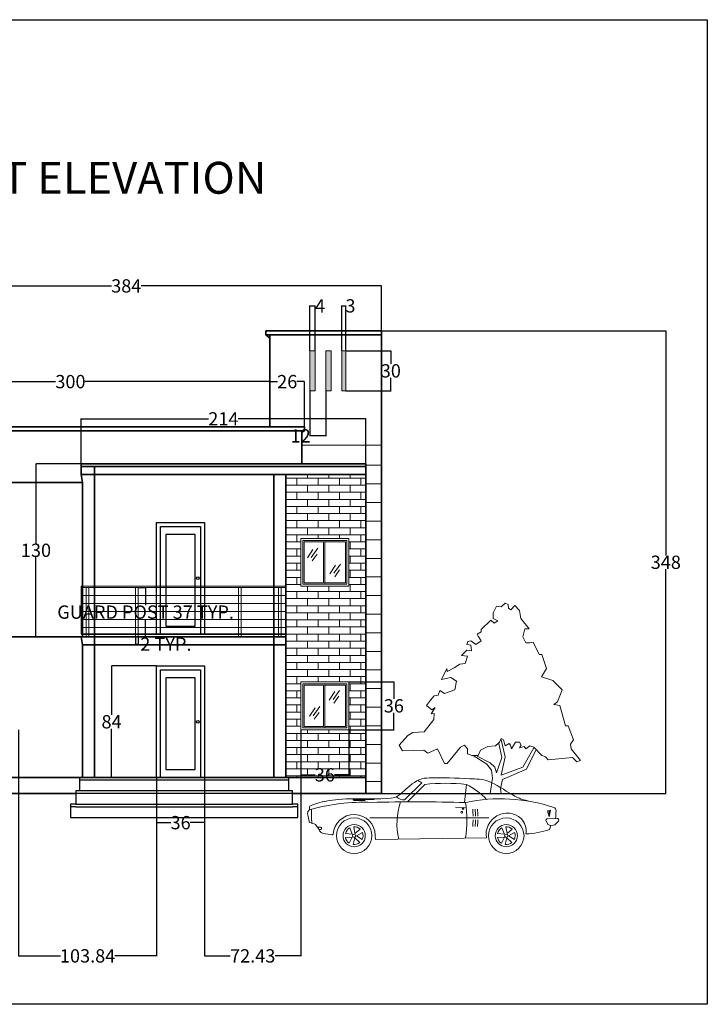
# Model space of a CAD drawing. Units: inches. Extents: x -16 to 1298, y 3 to 744.
# Tile 5 of 5: x 781 to 1298, y 3 to 744. Entities that reach past the tile are written whole.
import ezdxf

# ---------------------------------------------------------------- set-up
doc = ezdxf.new("R2010")
doc.units = ezdxf.units.IN
doc.header["$MEASUREMENT"] = 0
for name, color, linetype, lineweight in [('A-ANNO-DIMS', 2, 'Continuous', 18), ('A-ANNO-TITL', 7, 'Continuous', 35), ('A-DOOR', 3, 'Continuous', 25), ('A-ELEV', 7, 'Continuous', 35), ('A-ELEV-JNTS', 8, 'Continuous', 13), ('A-ELEV-VENT', 7, 'Continuous', 18), ('A-FLOR-HRAL', 4, 'Continuous', 18), ('A-FLOR-STRS', 7, 'Continuous', 25), ('A-GLAZ', 4, 'Continuous', 18), ('A-ROOF', 7, 'Continuous', 35), ('A-SITE-ENTG', 8, 'Continuous', 13), ('C-TOPO', 7, 'Continuous', 30), ('PLANT', 3, 'Continuous', 13)]:
    doc.layers.add(name, color=color, linetype=linetype, lineweight=lineweight)
doc.layers.add('A-ELEV-VENT-PATT', color=18, linetype='Continuous', lineweight=13, true_color=0x000000)
doc.layers.add('A-WALL-PATT', color=251, linetype='Continuous', lineweight=13, true_color=0x636466)
doc.styles.get("Standard").update_dxf_attribs({"font": 'arial.ttf'})
doc.dimstyles.get("Standard").update_dxf_attribs({"dimtxt": 10, "dimasz": 0.18, "dimexe": 0.18, "dimexo": 0.0625, "dimgap": 0.09, "dimtad": 0, "dimtih": 1, "dimtoh": 1, "dimdec": 0, "dimzin": 0, "dimdsep": 46, "dimlunit": 3, "dimtxsty": 'Standard', "dimcen": 0.09, "dimadec": 0, "dimazin": 0, "dimtfac": 1, "dimtdec": 0, "dimtofl": 0, "dimtmove": 0, "dimatfit": 3, "dimfxl": 1, "dimtolj": 1, "dimtzin": 0, "dimarcsym": 0})
pattern_1 = [(0, (565.852, -507.463), (0, 5.334), []), (90, (565.852, -507.463), (-8, 5.334), [5.334, -5.334])]

# ---------------------------------------------------------------- blocks, each defined once
blk = doc.blocks.new('*U12')
for p, q in [((1.5, 1.5), (1.5, 34.5)), ((1.5, 34.5), (18, 34.5)), ((18, 1.5), (18, 34.5)), ((18, 34.5), (34.5, 34.5)), ((34.5, 34.5), (34.5, 1.5)), ((18, 1.5), (1.5, 1.5)), ((34.5, 1.5), (18, 1.5))]:
    blk.add_line(p, q)
blk.add_lwpolyline([(0, 0), (0, 36), (36, 36), (36, 0)], close=True)
for points in [[(17, 33.5), (17, 2.5), (2.5, 2.5), (2.5, 33.5), (17, 33.5)], [(18, 33.5), (33.5, 33.5), (33.5, 2.5), (18, 2.5)]]:
    blk.add_lwpolyline(points)
blk = doc.blocks.new('*U16')
blk.add_lwpolyline([(3.12, 0.01), (0.12, 0.01), (0.12, 84.01), (36.12, 84.01), (36.12, 0.01), (33.12, 0.01)])
for points in [[(33.12, 80.99), (33.12, 0.01), (3.12, 0.01), (3.12, 80.99)], [(29.12, 6.01), (29.12, 74.99), (7.12, 74.99), (7.12, 6.01)]]:
    blk.add_lwpolyline(points, close=True)
blk.add_circle((31.12, 42.01), 1)
blk = doc.blocks.new('*U15')
blk.add_lwpolyline([(3.12, 0.01), (0.12, 0.01), (0.12, 84.01), (36.12, 84.01), (36.12, 0.01), (33.12, 0.01)])
for points in [[(33.12, 80.99), (33.12, 0.01), (3.12, 0.01), (3.12, 80.99)], [(29.12, 6.01), (29.12, 74.99), (7.12, 74.99), (7.12, 6.01)]]:
    blk.add_lwpolyline(points, close=True)
blk.add_circle((31.12, 42.01), 1)
blk = doc.blocks.new('Tree - type 3 evergreen elevation')
for points in [[(22.0124, 137.721), (18.5475, 141.5624), (15.5282, 138.2446), (13.8028, 139.3505), (13.3714, 142.1153), (11.2148, 143.2214), (8.1954, 140.4564), (4.7447, 141.0094), (2.1567, 136.0326), (2.1567, 131.6088), (5.6074, 129.9499), (3.0193, 128.2909), (0.4313, 130.5029), (-6.9015, 123.3141), (-6.9015, 121.6552), (-9.9208, 119.9963), (-9.0581, 118.3373), (-6.9015, 115.0195), (-10.7835, 112.2546), (-14.6656, 115.0195), (-16.8222, 114.4665), (-17.6849, 112.2546), (-14.6656, 111.7016), (-14.2342, 107.2778), (-17.6065, 107.8307), (-21.5669, 103.9599), (-17.2536, 103.4069), (-18.9789, 97.8771), (-22.8609, 97.3241), (-27.1743, 94.5593), (-32.3504, 91.7944), (-32.7817, 94.0063), (-36.6638, 85.7116), (-29.7624, 87.3705), (-25.449, 84.6056), (-26.743, 77.9699), (-34.507, 75.205), (-37.9578, 77.4169), (-39.2518, 74.099), (-42.2711, 73.5461), (-44.8592, 70.2282), (-47.8786, 66.3574), (-43.9965, 63.0395), (-41.4085, 64.6985), (-44.3346, 59.8898), (-42.2089, 60.1377), (-42.5159, 55.7849), (-49.6039, 46.4502), (-58.2307, 45.8972), (-62.1127, 43.6853), (-68.5828, 36.4966), (-65.9947, 32.0727), (-50.0352, 32.6257), (-47.0159, 30.4138), (-39.6831, 33.7317), (-34.507, 22.6721), (-32.3504, 22.6721), (-22.4296, 34.8376), (-19.4102, 36.4966), (-17.2536, 33.7317), (-17.2536, 29.8608), (-13.8028, 28.7549), (-9.0581, 28.7549), (-7.3328, 32.6257), (-1.7254, 35.3906), (3.8821, 35.9436), (6.4701, 38.1555), (6.9014, 38.7085), (8.1954, 41.4734), (9.9208, 40.3674), (11.2148, 35.9436), (14.2341, 37.6025), (15.0968, 36.4966), (15.9595, 33.7317), (18.9789, 38.7085), (21.9982, 38.7085), (23.2922, 36.4966), (21.9982, 34.2847), (25.4489, 35.3906), (26.743, 33.7317), (29.7623, 35.9436), (32.7817, 34.8376), (38.8204, 28.7549), (41.4084, 27.6489), (43.5651, 25.437), (61.6813, 27.0959), (65.132, 23.7781), (67.7201, 24.884), (60.8186, 33.7317), (60.3873, 37.0495), (62.544, 40.3674), (58.662, 50.874), (56.5053, 50.874), (52.1919, 66.3574), (47.8785, 66.9103), (50.4665, 69.1222), (53.9172, 77.9699), (47.0158, 85.1586), (38.3891, 87.9235), (42.2711, 94.0063)], [(42.2711, 94.0063), (38.8204, 104.5129), (36.6637, 104.5129), (32.3503, 113.9135), (29.7623, 113.3605), (26.743, 113.3605), (24.5862, 117.7844), (25.8802, 123.8671), (29.331, 123.8671), (22.8609, 131.6088), (21.9982, 137.6916)], [(-9.9208, 28.2019), (0, 23.2251), (3.4507, 19.9072), (4.7447, 15.4834), (8.6267, 27.0959), (6.4701, 37.6025)], [(8.1954, 40.3674), (11.2148, 27.6489), (8.1954, 13.8245), (24.5862, 19.9072), (32.7817, 34.2847)], [(34.5071, 33.1787), (27.1743, 18.2483), (9.0581, 10.5066), (7.7641, 3.8708), (8.1954, 0)], [(-12.9401, 28.7549), (-2.588, 22.1191), (0.8626, 17.6953), (1.7253, 11.6125), (0, 0)]]:
    blk.add_lwpolyline(points)
blk = doc.blocks.new('*U20')
for p, q in [((72.93, 40.23), (85.8, 53.18)), ((75, 38.82), (88.08, 51.97)), ((119.39, 51.91), (117.92, 38.32)), ((50.13, 41.06), (34.31, 40.98)), ((43.26, 39.85), (35.15, 39.78)), ((35.3, 40.46), (50.13, 40.62)), ((111.09, 34.73), (118.48, 34.64)), ((46.65, 26.83), (136.29, 26.77)), ((179.3, 24.35), (180.25, 22.49)), ((180.37, 26.17), (187.51, 26.41)), ((186.68, 22.17), (188.51, 24.37)), ((7.45, 19.78), (9.74, 19.8)), ((9.76, 17.93), (8.53, 17.92)), ((10.37, 19.19), (10.38, 18.56)), ((182.62, 21.14), (184.91, 21.28)), ((50.87, 13.52), (50.91, 10.52))]:
    blk.add_line(p, q)
for points in [[(35.31, 39.93), (35.3, 40.27, 0.269532), (35.14, 40.54), (34.38, 40.96, 0.575383), (34.15, 40.83), (34.15, 40.49, 0.269532), (34.32, 40.22), (35.08, 39.79, 0.575383)], [(28.49, 15.1), (33.61, 14.4), (31.65, 19.18, 0.199906)], [(34.64, 20.05), (35.56, 14.97), (39.5, 18.31, 0.199906)], [(41.25, 15.74), (36.7, 13.3), (41.09, 10.58, 0.199906)], [(142.85, 15.1), (147.96, 14.4), (146.01, 19.18, 0.199906)], [(148.99, 20.05), (149.91, 14.97), (153.85, 18.31, 0.199906)], [(155.6, 15.74), (151.06, 13.3), (155.45, 10.58, 0.199906)], [(31.31, 7.72), (33.55, 12.37), (28.4, 11.99, 0.199906)], [(39.19, 8.12), (35.46, 11.69), (34.23, 6.67, 0.199906)], [(145.66, 7.72), (147.9, 12.37), (142.75, 11.99, 0.199906)], [(153.54, 8.12), (149.81, 11.69), (148.59, 6.67, 0.199906)]]:
    blk.add_lwpolyline(points, format="xyb", close=True)
for points in [[(181.58, 27.46), (181.53, 31.95), (180.48, 32.43)], [(181.58, 27.46), (181.53, 31.95), (182.57, 32.45)], [(50.91, 10.52), (134.38, 11.83)]]:
    blk.add_lwpolyline(points)
for centre, radius in [((115.89, 31.01), 0.619), ((34.98, 13.35), 13.35), ((149.33, 13.35), 13.35), ((34.98, 13.35), 8.35), ((149.33, 13.35), 8.35), ((34.98, 13.35), 1.25), ((149.33, 13.35), 1.25)]:
    blk.add_circle(centre, radius)
for centre, radius, start, end in [((114.6, 105.09), 59.37, 237.61027, 240.97846), ((103.45, -95), 147.78, 83.81633, 95.97054), ((95.51, 3.91), 53.61, 43.27479, 63.56652), ((42.18, -111.35), 149.91, 87.83928, 105.80965), ((20.53, -3.15), 43.06, 98.53035, 116.11198), ((80.1, -1364.13), 1402.96, 88.42296, 91.3179), ((73.29, 50.49), 10.26, 230.42401, 268.00854), ((118.31, 22.51), 51.16, 161.43071, 193.23633), ((145.17, -84.88), 125.99, 71.52833, 102.12419), ((25.66, 24.94), 94.01, 351.8279, 8.16738), ((79.16, 30.11), 76.3, 177.57734, 185.52052), ((45.64, 26.83), 78.76, 0.85201, 4.65562), ((47.43, 26.85), 78.76, 0.85201, 4.65562), ((49.23, 26.87), 78.76, 0.85201, 4.65562), ((150.1, 14.36), 15.92, 49.2263, 189.1528), ((216.26, 37.76), 36.17, 188.46832, 196.53145), ((146.68, 36.98), 36.17, 344.74319, 352.80633), ((184.3, 32.25), 2.49, 357.93203, 71.52833), ((116.55, 34.7), 70.29, 353.19423, 357.93203), ((34.98, 13.35), 15.9, 0.63732, 176.34123), ((45.64, 26.83), 78.76, 355.26443, 358.86328), ((47.43, 26.85), 78.76, 355.26443, 358.86328), ((49.23, 26.87), 78.76, 355.26443, 358.86328), ((149.4, 16.55), 14.84, 352.72855, 41.66131), ((180.41, 24.92), 1.25, 91.93898, 207.10902), ((182.47, 23.63), 2.49, 207.10902, 273.46767), ((187.55, 25.16), 1.25, 320.16835, 91.93898), ((9.75, 19.18), 0.623, 0.63732, 90.63732), ((9.76, 18.55), 0.623, 270.63732, 0.63732), ((162.47, 70.82), 56.18, 271.6865, 290.2774), ((114.25, 37.03), 70.29, 344.3985, 346.93849), ((184.76, 23.76), 2.49, 273.46767, 320.16835)]:
    blk.add_arc(centre, radius, start, end)
blk.add_ellipse((116.89, 33.59), major_axis=(-0.63, -0.007), ratio=0.610043)
for points, knots in [([(11.39, 38.92), (18.06, 40.19), (30.91, 42.01), (64.77, 40.11), (70.25, 44.91), (82.35, 56.38), (99.18, 57.3), (116.06, 56.35), (133.04, 55.87), (145.24, 49.87), (153.62, 43.8), (161.17, 40.68), (164.92, 39.73), (167.29, 39.15)], [18.629823, 18.629823, 18.629823, 18.629823, 19.527405, 20.700571, 21.107983, 21.608568, 21.92336, 23.151359, 23.716171, 23.908743, 24.77794, 24.943072, 25.187755, 25.187755, 25.187755, 25.187755]), ([(19.11, 14.36), (18.99, 14.21), (18.5, 13.81), (15.35, 15), (9.19, 13.94), (7.26, 22.22), (3.01, 22.66), (1.32, 23.61), (0.64, 26.92), (-0.96, 31.49), (1.54, 32.64), (1.5, 34.06), (1.49, 34.8), (1.49, 35.06), (1.52, 35.3), (1.58, 35.51)], [16.815853, 16.815853, 16.815853, 16.815853, 16.838212, 16.885395, 17.18439, 17.479846, 17.654423, 17.670693, 17.696923, 18.016358, 18.052739, 18.140805, 18.140805, 18.140805, 18.172382, 18.172382, 18.172382, 18.172382])]:
    blk.add_open_spline(points, degree=3, knots=knots)
blk = doc.blocks.new('GLASS-REFLECTION-SMALL')
for p, q in [((4.25, 8.64), (0, 2.2)), ((7.92, 9.52), (2.93, 2.64)), ((7.33, 5.13), (3.66, 0))]:
    blk.add_line(p, q)
blk = doc.blocks.new('BALCONY-GUARD-POST')
for p, q in [((0, 37), (0, 0)), ((2, 37), (2, 0))]:
    blk.add_line(p, q)
blk = doc.blocks.new('*D38')
at = {"layer": 'A-ANNO-DIMS', "color": 0, "lineweight": -2, "transparency": 16777216}
for p, q in [((870.56, 316.99), (876.23, 316.99)), ((876.05, 316.81), (876.05, 303.76)), ((876.05, 280.17), (876.05, 293.22)), ((870.56, 279.99), (876.23, 279.99))]:
    blk.add_line(p, q, dxfattribs=at)
at = {"layer": 'A-ANNO-DIMS', "color": 0, "transparency": 16777216}
for points in [[(876.02, 316.81), (876.08, 316.81), (876.05, 316.99)], [(876.02, 280.17), (876.08, 280.17), (876.05, 279.99)]]:
    blk.add_solid(points, dxfattribs=at)
at = {"layer": 'Defpoints', "color": 0, "transparency": 16777216}
for p in [(870.5, 316.99), (876.05, 316.99), (870.5, 279.99)]:
    blk.add_point(p, dxfattribs=at)
at = {"layer": 'A-ANNO-DIMS', "color": 0, "transparency": 16777216, "insert": (876.05, 298.49), "char_height": 10, "attachment_point": 5}
blk.add_mtext('\\A1;GUARD POST 37 TYP.', dxfattribs=at)
blk = doc.blocks.new('*D39')
at = {"layer": 'A-ANNO-DIMS', "color": 0, "lineweight": -2, "transparency": 16777216}
for p, q in [((868.5, 279.93), (868.5, 274.26)), ((868.68, 274.44), (870.32, 274.44)), ((870.5, 279.93), (870.5, 274.26)), ((870.5, 274.44), (870.68, 274.44))]:
    blk.add_line(p, q, dxfattribs=at)
at = {"layer": 'A-ANNO-DIMS', "color": 0, "transparency": 16777216}
for points in [[(868.68, 274.47), (868.68, 274.41), (868.5, 274.44)], [(870.32, 274.47), (870.32, 274.41), (870.5, 274.44)]]:
    blk.add_solid(points, dxfattribs=at)
at = {"layer": 'Defpoints', "color": 0, "transparency": 16777216}
for p in [(868.5, 279.99), (870.5, 279.99), (870.5, 274.44)]:
    blk.add_point(p, dxfattribs=at)
at = {"layer": 'A-ANNO-DIMS', "color": 0, "transparency": 16777216, "insert": (891.31, 274.44), "char_height": 10, "attachment_point": 5}
blk.add_mtext('\\A1;2 TYP.', dxfattribs=at)
blk = doc.blocks.new('*D63')
at = {"layer": 'A-ANNO-DIMS', "color": 0, "lineweight": -2, "transparency": 16777216}
for p, q in [((669.53, 438.05), (669.53, 544.07)), ((669.71, 543.89), (850.42, 543.89)), ((1053.35, 543.89), (872.64, 543.89)), ((1053.53, 510.05), (1053.53, 544.07))]:
    blk.add_line(p, q, dxfattribs=at)
at = {"layer": 'A-ANNO-DIMS', "color": 0, "transparency": 16777216}
for points in [[(669.71, 543.92), (669.71, 543.86), (669.53, 543.89)], [(1053.35, 543.92), (1053.35, 543.86), (1053.53, 543.89)]]:
    blk.add_solid(points, dxfattribs=at)
at = {"layer": 'Defpoints', "color": 0, "transparency": 16777216}
for p in [(1053.53, 543.89), (1053.53, 509.99), (669.53, 437.99)]:
    blk.add_point(p, dxfattribs=at)
at = {"layer": 'A-ANNO-DIMS', "color": 0, "transparency": 16777216, "insert": (861.53, 543.89), "char_height": 10, "attachment_point": 5}
blk.add_mtext('\\A1;384', dxfattribs=at)
blk = doc.blocks.new('*D64')
at = {"layer": 'A-ANNO-DIMS', "color": 0, "lineweight": -2, "transparency": 16777216}
for p, q in [((1053.59, 509.99), (1267.34, 509.99)), ((1267.16, 509.81), (1267.16, 341.19)), ((1267.16, 162.17), (1267.16, 330.79)), ((1053.59, 161.99), (1267.34, 161.99))]:
    blk.add_line(p, q, dxfattribs=at)
at = {"layer": 'A-ANNO-DIMS', "color": 0, "transparency": 16777216}
for points in [[(1267.13, 509.81), (1267.19, 509.81), (1267.16, 509.99)], [(1267.13, 162.17), (1267.19, 162.17), (1267.16, 161.99)]]:
    blk.add_solid(points, dxfattribs=at)
at = {"layer": 'Defpoints', "color": 0, "transparency": 16777216}
for p in [(1053.53, 509.99), (1267.16, 509.99), (1053.53, 161.99)]:
    blk.add_point(p, dxfattribs=at)
at = {"layer": 'A-ANNO-DIMS', "color": 0, "transparency": 16777216, "insert": (1267.16, 335.99), "char_height": 10, "attachment_point": 5}
blk.add_mtext('\\A1;348', dxfattribs=at)
blk = doc.blocks.new('*D71')
at = {"layer": 'A-ANNO-DIMS', "color": 0, "lineweight": -2, "transparency": 16777216}
for p, q in [((827.47, 409.99), (793.45, 409.99)), ((793.63, 409.81), (793.63, 350.19)), ((793.63, 280.17), (793.63, 339.79)), ((827.47, 279.99), (793.45, 279.99))]:
    blk.add_line(p, q, dxfattribs=at)
at = {"layer": 'A-ANNO-DIMS', "color": 0, "transparency": 16777216}
for points in [[(793.6, 409.81), (793.66, 409.81), (793.63, 409.99)], [(793.6, 280.17), (793.66, 280.17), (793.63, 279.99)]]:
    blk.add_solid(points, dxfattribs=at)
at = {"layer": 'Defpoints', "color": 0, "transparency": 16777216}
for p in [(793.63, 409.99), (827.53, 409.99), (827.53, 279.99)]:
    blk.add_point(p, dxfattribs=at)
at = {"layer": 'A-ANNO-DIMS', "color": 0, "transparency": 16777216, "insert": (793.63, 344.99), "char_height": 10, "attachment_point": 5}
blk.add_mtext('\\A1;130', dxfattribs=at)
blk = doc.blocks.new('*D74')
at = {"layer": 'A-ANNO-DIMS', "color": 0, "lineweight": -2, "transparency": 16777216}
for p, q in [((780.53, 209.93), (780.53, 39.71)), ((884.37, 173.94), (884.37, 39.71)), ((780.71, 39.89), (812.09, 39.89)), ((884.19, 39.89), (852.8, 39.89))]:
    blk.add_line(p, q, dxfattribs=at)
at = {"layer": 'A-ANNO-DIMS', "color": 0, "transparency": 16777216}
for points in [[(780.71, 39.92), (780.71, 39.86), (780.53, 39.89)], [(884.19, 39.92), (884.19, 39.86), (884.37, 39.89)]]:
    blk.add_solid(points, dxfattribs=at)
at = {"layer": 'Defpoints', "color": 0, "transparency": 16777216}
for p in [(780.53, 209.99), (884.37, 174), (884.37, 39.89)]:
    blk.add_point(p, dxfattribs=at)
at = {"layer": 'A-ANNO-DIMS', "color": 0, "transparency": 16777216, "insert": (832.45, 39.89), "char_height": 10, "attachment_point": 5}
blk.add_mtext('\\A1;103.84', dxfattribs=at)
blk = doc.blocks.new('*D75')
at = {"layer": 'A-ANNO-DIMS', "color": 0, "lineweight": -2, "transparency": 16777216}
for p, q in [((884.37, 173.94), (884.37, 139.92)), ((920.37, 173.94), (920.37, 139.92)), ((884.55, 140.1), (895.12, 140.1)), ((920.19, 140.1), (909.61, 140.1))]:
    blk.add_line(p, q, dxfattribs=at)
at = {"layer": 'A-ANNO-DIMS', "color": 0, "transparency": 16777216}
for points in [[(884.55, 140.13), (884.55, 140.07), (884.37, 140.1)], [(920.19, 140.13), (920.19, 140.07), (920.37, 140.1)]]:
    blk.add_solid(points, dxfattribs=at)
at = {"layer": 'Defpoints', "color": 0, "transparency": 16777216}
for p in [(884.37, 174), (920.37, 174), (884.37, 140.1)]:
    blk.add_point(p, dxfattribs=at)
at = {"layer": 'A-ANNO-DIMS', "color": 0, "transparency": 16777216, "insert": (902.37, 140.1), "char_height": 10, "attachment_point": 5}
blk.add_mtext('\\A1;36', dxfattribs=at)
blk = doc.blocks.new('*D76')
at = {"layer": 'A-ANNO-DIMS', "color": 0, "lineweight": -2, "transparency": 16777216}
for p, q in [((884.31, 258), (850.29, 258)), ((850.47, 257.82), (850.47, 221.2)), ((850.47, 174.18), (850.47, 210.81)), ((884.31, 174), (850.29, 174))]:
    blk.add_line(p, q, dxfattribs=at)
at = {"layer": 'A-ANNO-DIMS', "color": 0, "transparency": 16777216}
for points in [[(850.44, 257.82), (850.5, 257.82), (850.47, 258)], [(850.44, 174.18), (850.5, 174.18), (850.47, 174)]]:
    blk.add_solid(points, dxfattribs=at)
at = {"layer": 'Defpoints', "color": 0, "transparency": 16777216}
for p in [(850.47, 258), (884.37, 258), (884.37, 174)]:
    blk.add_point(p, dxfattribs=at)
at = {"layer": 'A-ANNO-DIMS', "color": 0, "transparency": 16777216, "insert": (850.47, 216), "char_height": 10, "attachment_point": 5}
blk.add_mtext('\\A1;84', dxfattribs=at)
blk = doc.blocks.new('*D77')
at = {"layer": 'A-ANNO-DIMS', "color": 0, "lineweight": -2, "transparency": 16777216}
for p, q in [((992.79, 209.93), (992.79, 39.71)), ((920.37, 173.94), (920.37, 39.71)), ((920.55, 39.89), (939.66, 39.89)), ((992.61, 39.89), (973.5, 39.89))]:
    blk.add_line(p, q, dxfattribs=at)
at = {"layer": 'A-ANNO-DIMS', "color": 0, "transparency": 16777216}
for points in [[(920.55, 39.92), (920.55, 39.86), (920.37, 39.89)], [(992.61, 39.92), (992.61, 39.86), (992.79, 39.89)]]:
    blk.add_solid(points, dxfattribs=at)
at = {"layer": 'Defpoints', "color": 0, "transparency": 16777216}
for p in [(992.79, 209.99), (920.37, 174), (992.79, 39.89)]:
    blk.add_point(p, dxfattribs=at)
at = {"layer": 'A-ANNO-DIMS', "color": 0, "transparency": 16777216, "insert": (956.58, 39.89), "char_height": 10, "attachment_point": 5}
blk.add_mtext('\\A1;72.43', dxfattribs=at)
blk = doc.blocks.new('*D78')
at = {"layer": 'A-ANNO-DIMS', "color": 0, "lineweight": -2, "transparency": 16777216}
for p, q in [((992.79, 209.93), (992.79, 175.91)), ((1028.79, 209.93), (1028.79, 175.91)), ((992.97, 176.09), (1003.55, 176.09)), ((1028.61, 176.09), (1018.04, 176.09))]:
    blk.add_line(p, q, dxfattribs=at)
at = {"layer": 'A-ANNO-DIMS', "color": 0, "transparency": 16777216}
for points in [[(992.97, 176.12), (992.97, 176.06), (992.79, 176.09)], [(1028.61, 176.12), (1028.61, 176.06), (1028.79, 176.09)]]:
    blk.add_solid(points, dxfattribs=at)
at = {"layer": 'Defpoints', "color": 0, "transparency": 16777216}
for p in [(992.79, 209.99), (1028.79, 209.99), (992.79, 176.09)]:
    blk.add_point(p, dxfattribs=at)
at = {"layer": 'A-ANNO-DIMS', "color": 0, "transparency": 16777216, "insert": (1010.79, 176.09), "char_height": 10, "attachment_point": 5}
blk.add_mtext('\\A1;36', dxfattribs=at)
blk = doc.blocks.new('*D79')
at = {"layer": 'A-ANNO-DIMS', "color": 0, "lineweight": -2, "transparency": 16777216}
for p, q in [((1028.86, 245.99), (1062.87, 245.99)), ((1062.69, 245.81), (1062.69, 233.19)), ((1062.69, 210.17), (1062.69, 222.79)), ((1028.86, 209.99), (1062.87, 209.99))]:
    blk.add_line(p, q, dxfattribs=at)
at = {"layer": 'A-ANNO-DIMS', "color": 0, "transparency": 16777216}
for points in [[(1062.66, 245.81), (1062.72, 245.81), (1062.69, 245.99)], [(1062.66, 210.17), (1062.72, 210.17), (1062.69, 209.99)]]:
    blk.add_solid(points, dxfattribs=at)
at = {"layer": 'Defpoints', "color": 0, "transparency": 16777216}
for p in [(1028.79, 245.99), (1028.79, 209.99), (1062.69, 209.99)]:
    blk.add_point(p, dxfattribs=at)
at = {"layer": 'A-ANNO-DIMS', "color": 0, "transparency": 16777216, "insert": (1062.69, 227.99), "char_height": 10, "attachment_point": 5}
blk.add_mtext('\\A1;36', dxfattribs=at)
blk = doc.blocks.new('*D80')
at = {"layer": 'A-ANNO-DIMS', "color": 0, "lineweight": -2, "transparency": 16777216}
for p, q in [((827.53, 410.05), (827.53, 444.07)), ((827.71, 443.89), (923.33, 443.89)), ((1041.35, 443.89), (945.73, 443.89)), ((1041.53, 410.05), (1041.53, 444.07))]:
    blk.add_line(p, q, dxfattribs=at)
at = {"layer": 'A-ANNO-DIMS', "color": 0, "transparency": 16777216}
for points in [[(827.71, 443.92), (827.71, 443.86), (827.53, 443.89)], [(1041.35, 443.92), (1041.35, 443.86), (1041.53, 443.89)]]:
    blk.add_solid(points, dxfattribs=at)
at = {"layer": 'Defpoints', "color": 0, "transparency": 16777216}
for p in [(1041.53, 443.89), (827.53, 409.99), (1041.53, 409.99)]:
    blk.add_point(p, dxfattribs=at)
at = {"layer": 'A-ANNO-DIMS', "color": 0, "transparency": 16777216, "insert": (934.53, 443.89), "char_height": 10, "attachment_point": 5}
blk.add_mtext('\\A1;214', dxfattribs=at)
blk = doc.blocks.new('*D81')
at = {"layer": 'A-ANNO-DIMS', "color": 0, "lineweight": -2, "transparency": 16777216}
for p, q in [((669.53, 438.05), (669.53, 472.07)), ((669.71, 471.89), (808.41, 471.89)), ((969.35, 471.89), (830.65, 471.89)), ((969.53, 438.05), (969.53, 472.07))]:
    blk.add_line(p, q, dxfattribs=at)
at = {"layer": 'A-ANNO-DIMS', "color": 0, "transparency": 16777216}
for points in [[(669.71, 471.92), (669.71, 471.86), (669.53, 471.89)], [(969.35, 471.92), (969.35, 471.86), (969.53, 471.89)]]:
    blk.add_solid(points, dxfattribs=at)
at = {"layer": 'Defpoints', "color": 0, "transparency": 16777216}
for p in [(969.53, 471.89), (669.53, 437.99), (969.53, 437.99)]:
    blk.add_point(p, dxfattribs=at)
at = {"layer": 'A-ANNO-DIMS', "color": 0, "transparency": 16777216, "insert": (819.53, 471.89), "char_height": 10, "attachment_point": 5}
blk.add_mtext('\\A1;300', dxfattribs=at)
blk = doc.blocks.new('*D82')
at = {"layer": 'A-ANNO-DIMS', "color": 0, "lineweight": -2, "transparency": 16777216}
for p, q in [((969.53, 438.05), (969.53, 472.07)), ((969.71, 471.89), (975.19, 471.89)), ((995.35, 471.89), (989.86, 471.89)), ((995.53, 438.05), (995.53, 472.07))]:
    blk.add_line(p, q, dxfattribs=at)
at = {"layer": 'A-ANNO-DIMS', "color": 0, "transparency": 16777216}
for points in [[(969.71, 471.92), (969.71, 471.86), (969.53, 471.89)], [(995.35, 471.92), (995.35, 471.86), (995.53, 471.89)]]:
    blk.add_solid(points, dxfattribs=at)
at = {"layer": 'Defpoints', "color": 0, "transparency": 16777216}
for p in [(995.53, 471.89), (969.53, 437.99), (995.53, 437.99)]:
    blk.add_point(p, dxfattribs=at)
at = {"layer": 'A-ANNO-DIMS', "color": 0, "transparency": 16777216, "insert": (982.53, 471.89), "char_height": 10, "attachment_point": 5}
blk.add_mtext('\\A1;26', dxfattribs=at)
blk = doc.blocks.new('*D83')
at = {"layer": 'A-ANNO-DIMS', "color": 0, "lineweight": -2, "transparency": 16777216}
for p, q in [((1026.59, 494.99), (1060.61, 494.99)), ((1060.43, 494.81), (1060.43, 485.19)), ((1060.43, 465.17), (1060.43, 474.79)), ((1026.59, 464.99), (1060.61, 464.99))]:
    blk.add_line(p, q, dxfattribs=at)
at = {"layer": 'A-ANNO-DIMS', "color": 0, "transparency": 16777216}
for points in [[(1060.4, 494.81), (1060.46, 494.81), (1060.43, 494.99)], [(1060.4, 465.17), (1060.46, 465.17), (1060.43, 464.99)]]:
    blk.add_solid(points, dxfattribs=at)
at = {"layer": 'Defpoints', "color": 0, "transparency": 16777216}
for p in [(1026.53, 494.99), (1026.53, 464.99), (1060.43, 464.99)]:
    blk.add_point(p, dxfattribs=at)
at = {"layer": 'A-ANNO-DIMS', "color": 0, "transparency": 16777216, "insert": (1060.43, 479.99), "char_height": 10, "attachment_point": 5}
blk.add_mtext('\\A1;30', dxfattribs=at)
blk = doc.blocks.new('*D84')
at = {"layer": 'A-ANNO-DIMS', "color": 0, "lineweight": -2, "transparency": 16777216}
for p, q in [((999.53, 495.05), (999.53, 529.07)), ((999.71, 528.89), (1003.35, 528.89)), ((1003.53, 495.05), (1003.53, 529.07)), ((1003.53, 528.89), (1003.71, 528.89))]:
    blk.add_line(p, q, dxfattribs=at)
at = {"layer": 'A-ANNO-DIMS', "color": 0, "transparency": 16777216}
for points in [[(999.71, 528.92), (999.71, 528.86), (999.53, 528.89)], [(1003.35, 528.92), (1003.35, 528.86), (1003.53, 528.89)]]:
    blk.add_solid(points, dxfattribs=at)
at = {"layer": 'Defpoints', "color": 0, "transparency": 16777216}
for p in [(1003.53, 528.89), (999.53, 494.99), (1003.53, 494.99)]:
    blk.add_point(p, dxfattribs=at)
at = {"layer": 'A-ANNO-DIMS', "color": 0, "transparency": 16777216, "insert": (1007.26, 528.89), "char_height": 10, "attachment_point": 5}
blk.add_mtext('\\A1;4', dxfattribs=at)
blk = doc.blocks.new('*D85')
at = {"layer": 'A-ANNO-DIMS', "color": 0, "lineweight": -2, "transparency": 16777216}
for p, q in [((1023.53, 495.05), (1023.53, 529.07)), ((1023.71, 528.89), (1026.35, 528.89)), ((1026.53, 495.05), (1026.53, 529.07)), ((1026.53, 528.89), (1026.71, 528.89))]:
    blk.add_line(p, q, dxfattribs=at)
at = {"layer": 'A-ANNO-DIMS', "color": 0, "transparency": 16777216}
for points in [[(1023.71, 528.92), (1023.71, 528.86), (1023.53, 528.89)], [(1026.35, 528.92), (1026.35, 528.86), (1026.53, 528.89)]]:
    blk.add_solid(points, dxfattribs=at)
at = {"layer": 'Defpoints', "color": 0, "transparency": 16777216}
for p in [(1026.53, 528.89), (1023.53, 494.99), (1026.53, 494.99)]:
    blk.add_point(p, dxfattribs=at)
at = {"layer": 'A-ANNO-DIMS', "color": 0, "transparency": 16777216, "insert": (1030.07, 528.89), "char_height": 10, "attachment_point": 5}
blk.add_mtext('\\A1;3', dxfattribs=at)
blk = doc.blocks.new('*D86')
at = {"layer": 'A-ANNO-DIMS', "color": 0, "lineweight": -2, "transparency": 16777216}
for p, q in [((999.53, 464.93), (999.53, 430.91)), ((1011.53, 464.93), (1011.53, 430.91)), ((999.53, 431.09), (999.35, 431.09)), ((1011.35, 431.09), (999.71, 431.09))]:
    blk.add_line(p, q, dxfattribs=at)
at = {"layer": 'A-ANNO-DIMS', "color": 0, "transparency": 16777216}
for points in [[(999.71, 431.12), (999.71, 431.06), (999.53, 431.09)], [(1011.35, 431.12), (1011.35, 431.06), (1011.53, 431.09)]]:
    blk.add_solid(points, dxfattribs=at)
at = {"layer": 'Defpoints', "color": 0, "transparency": 16777216}
for p in [(999.53, 464.99), (1011.53, 464.99), (999.53, 431.09)]:
    blk.add_point(p, dxfattribs=at)
at = {"layer": 'A-ANNO-DIMS', "color": 0, "transparency": 16777216, "insert": (992.62, 431.09), "char_height": 10, "attachment_point": 5}
blk.add_mtext('\\A1;12', dxfattribs=at)

msp = doc.modelspace()

# ---------------------------------------------------------------- hatches: boundary and pattern name
at = {"layer": 'A-ELEV-VENT-PATT'}
h = msp.add_hatch(color=256, dxfattribs=at)
h.dxf.hatch_style = 1
h.paths.add_polyline_path([(1023.5287, 464.9884), (1026.5287, 464.9884), (1026.5287, 494.9884), (1023.5287, 494.9884)])
h.paths.add_polyline_path([(1011.5287, 464.9884), (1015.5287, 464.9884), (1015.5287, 494.9884), (1011.5287, 494.9884)])
h.paths.add_polyline_path([(1003.5287, 494.9884), (999.5287, 494.9884), (999.5287, 464.9884), (1003.5287, 464.9884)])
at = {"layer": 'A-WALL-PATT'}
h = msp.add_hatch(dxfattribs=at)
h.set_pattern_fill('AR-BRSTD', color=256, scale=2)
h.set_pattern_definition(pattern_1)
h.paths.add_polyline_path([(981.5287, 173.9884), (983.5287, 173.9884), (1041.5287, 173.9884), (1041.5287, 401.9884), (981.5287, 401.9884)])
h.paths.add_polyline_path([(992.7927, 317.9884), (992.7927, 353.9884), (1028.7927, 353.9884), (1028.7927, 317.9884)], flags=16)
h.paths.add_polyline_path([(994.2927, 319.4884), (994.2927, 352.4884), (1010.7927, 352.4884), (1027.2927, 352.4884), (1027.2927, 319.4884), (1010.7927, 319.4884)], flags=0)
h.paths.add_polyline_path([(1009.7927, 320.4884), (1009.7927, 351.4884), (995.2927, 351.4884), (995.2927, 320.4884)], flags=0)
h.paths.add_polyline_path([(1010.7927, 351.4884), (1026.2927, 351.4884), (1026.2927, 320.4884), (1010.7927, 320.4884)], flags=0)
h.paths.add_polyline_path([(1028.7927, 245.9884), (1028.7927, 209.9884), (992.7927, 209.9884), (992.7927, 245.9884)], flags=16)
h.paths.add_polyline_path([(1010.7927, 244.4884), (1027.2927, 244.4884), (1027.2927, 211.4884), (1010.7927, 211.4884), (994.2927, 211.4884), (994.2927, 244.4884)], flags=0)
h.paths.add_polyline_path([(1009.7927, 212.4884), (1009.7927, 243.4884), (995.2927, 243.4884), (995.2927, 212.4884)], flags=0)
h.paths.add_polyline_path([(1026.2927, 243.4884), (1026.2927, 212.4884), (1010.7927, 212.4884), (1010.7927, 243.4884)], flags=0)
h = msp.add_hatch(dxfattribs=at)
h.set_pattern_fill('AR-BRSTD', color=256, scale=2)
h.set_pattern_definition(pattern_1)
h.paths.add_polyline_path([(1041.5287, 273.9884), (981.5287, 273.9884), (981.5287, 173.9884), (983.5287, 173.9884), (1041.5287, 173.9884)])
h.paths.add_polyline_path([(1028.7927, 245.9884), (1028.7927, 209.9884), (992.7927, 209.9884), (992.7927, 245.9884)], flags=16)
h.paths.add_polyline_path([(1027.2927, 244.4884), (1027.2927, 211.4884), (1010.7927, 211.4884), (994.2927, 211.4884), (994.2927, 244.4884), (1010.7927, 244.4884)], flags=0)
h.paths.add_polyline_path([(1010.7927, 243.4884), (1026.2927, 243.4884), (1026.2927, 212.4884), (1010.7927, 212.4884)], flags=0)
h.paths.add_polyline_path([(1009.7927, 212.4884), (995.2927, 212.4884), (995.2927, 243.4884), (1009.7927, 243.4884)], flags=0)

# ---------------------------------------------------------------- linework, layer by layer
at = {"layer": 'A-ELEV'}
for p, q in [((1053.5287, 161.9884), (1053.5287, 509.9884)), ((1041.5287, 409.9884), (827.5287, 409.9884)), ((828.5287, 409.9884), (827.5287, 409.9884)), ((827.5287, 409.9884), (827.5287, 401.9884)), ((1041.5287, 407.9884), (827.5287, 407.9884)), ((837.5287, 173.9884), (837.5287, 407.9884)), ((1041.5287, 173.9884), (1041.5287, 409.9884)), ((1041.5287, 161.9884), (1041.5287, 409.9884)), ((1041.5287, 401.9884), (827.5287, 401.9884)), ((827.5287, 401.9884), (828.5287, 395.9884)), ((972.5287, 173.9884), (972.5287, 401.9884)), ((981.5287, 173.9884), (981.5287, 401.9884)), ((828.5287, 395.9884), (669.5287, 395.9884)), ((828.5287, 279.9884), (828.5287, 395.9884)), ((981.5287, 281.9884), (827.5287, 281.9884)), ((827.5287, 279.9884), (669.5287, 279.9884)), ((981.5287, 279.9884), (827.5287, 279.9884)), ((827.5287, 279.9884), (828.5287, 273.9884)), ((828.5287, 173.9884), (828.5287, 273.9884)), ((981.5287, 273.9884), (828.5287, 273.9884)), ((1041.5287, 173.9884), (669.5287, 173.9884)), ((972.5287, 173.9884), (981.5287, 173.9884)), ((981.5287, 173.9884), (981.5287, 173.9884)), ((823.5287, 161.9884), (669.5287, 161.9884)), ((1053.5287, 161.9884), (986.5287, 161.9884))]:
    msp.add_line(p, q, dxfattribs=at)
at = {"layer": 'A-ELEV-JNTS'}
for p, q in [((993.5287, 423.9884), (1053.5287, 423.9884)), ((1041.5287, 408.9515), (1053.5287, 408.9515)), ((1041.5287, 394.9515), (1053.5287, 394.9515)), ((1041.5287, 380.9515), (1053.5287, 380.9515)), ((1041.5287, 366.9515), (1053.5287, 366.9515)), ((1041.5287, 352.9515), (1053.5287, 352.9515)), ((1041.5287, 338.9515), (1053.5287, 338.9515)), ((1041.5287, 324.9515), (1053.5287, 324.9515)), ((1041.5287, 310.9515), (1053.5287, 310.9515)), ((1041.5287, 296.9515), (1053.5287, 296.9515)), ((1041.5287, 282.9515), (1053.5287, 282.9515)), ((1041.5287, 268.9515), (1053.5287, 268.9515)), ((1041.5287, 254.9515), (1053.5287, 254.9515)), ((1041.5287, 240.9515), (1053.5287, 240.9515)), ((1041.5287, 226.9515), (1053.5287, 226.9515)), ((1041.5287, 212.9515), (1053.5287, 212.9515)), ((1041.5287, 198.9515), (1053.5287, 198.9515)), ((1041.5287, 184.9515), (1053.5287, 184.9515)), ((1041.5287, 170.9515), (1053.5287, 170.9515))]:
    msp.add_line(p, q, dxfattribs=at)
at = {"layer": 'A-ELEV-VENT'}
for p, q in [((999.5287, 464.9884), (999.5287, 494.9884)), ((1003.5287, 494.9884), (999.5287, 494.9884)), ((1003.5287, 464.9884), (1003.5287, 494.9884)), ((1011.5287, 464.9884), (1011.5287, 494.9884)), ((1015.5287, 494.9884), (1011.5287, 494.9884)), ((1015.5287, 464.9884), (1015.5287, 494.9884)), ((1023.5287, 464.9884), (1023.5287, 494.9884)), ((1026.5287, 494.9884), (1023.5287, 494.9884)), ((1026.5287, 464.9884), (1026.5287, 494.9884)), ((1003.5287, 464.9884), (999.5287, 464.9884)), ((1015.5287, 464.9884), (1011.5287, 464.9884)), ((1026.5287, 464.9884), (1023.5287, 464.9884))]:
    msp.add_line(p, q, dxfattribs=at)
at = {"layer": 'A-FLOR-HRAL'}
for p, q in [((981.5287, 317.9884), (827.5287, 317.9884)), ((827.5287, 317.9884), (827.5287, 281.9884)), ((981.5287, 316.9884), (827.5287, 316.9884)), ((981.5287, 310.9884), (827.5287, 310.9884)), ((981.5287, 304.9884), (827.5287, 304.9884)), ((981.5287, 298.9884), (827.5287, 298.9884)), ((981.5287, 292.9884), (827.5287, 292.9884)), ((981.5287, 286.9884), (827.5287, 286.9884))]:
    msp.add_line(p, q, dxfattribs=at)
at = {"layer": 'A-FLOR-STRS'}
for p, q in [((826.5287, 163.9884), (826.5287, 173.9884)), ((983.5287, 171.9884), (826.5287, 171.9884)), ((981.5287, 173.9884), (983.5287, 173.9884)), ((983.5287, 173.9884), (983.5287, 163.9884)), ((826.5287, 163.9884), (823.5287, 163.9884)), ((823.5287, 163.9884), (823.5287, 153.9884)), ((828.5287, 163.9884), (826.5287, 163.9884)), ((983.5287, 163.9884), (828.5287, 163.9884)), ((986.5287, 163.9884), (983.5287, 163.9884)), ((986.5287, 153.9884), (986.5287, 163.9884)), ((826.5287, 161.9884), (823.5287, 161.9884)), ((828.5287, 161.9884), (826.5287, 161.9884)), ((983.5287, 161.9884), (828.5287, 161.9884)), ((986.5287, 161.9884), (983.5287, 161.9884)), ((823.5287, 153.9884), (819.5287, 153.9884)), ((819.5287, 153.9884), (819.5287, 143.9884)), ((823.5287, 151.9884), (819.5287, 151.9884)), ((823.5287, 153.9884), (983.5287, 153.9884)), ((823.5287, 151.9884), (983.5287, 151.9884)), ((983.5287, 153.9884), (986.5287, 153.9884)), ((983.5287, 151.9884), (986.5287, 151.9884)), ((990.5287, 153.9884), (986.5287, 153.9884)), ((990.5287, 151.9884), (986.5287, 151.9884)), ((990.5287, 143.9884), (990.5287, 153.9884)), ((819.5287, 143.9884), (986.5287, 143.9884)), ((986.5287, 143.9884), (990.5287, 143.9884))]:
    msp.add_line(p, q, dxfattribs=at)
at = {"layer": 'A-ROOF'}
for p, q in [((969.5287, 509.9884), (966.5287, 509.9884)), ((966.5287, 509.9884), (966.5287, 506.9884)), ((966.5287, 506.9884), (969.5287, 506.9884)), ((966.5287, 506.9884), (969.5287, 504.6453)), ((1053.5287, 509.9884), (969.5287, 509.9884)), ((969.5287, 437.9884), (969.5287, 506.9884)), ((1053.5287, 506.9884), (969.5287, 506.9884)), ((993.5287, 437.9884), (669.5287, 437.9884)), ((969.5287, 437.9884), (993.5287, 437.9884)), ((993.5287, 437.9884), (995.5287, 437.9884)), ((995.5287, 437.9884), (995.5287, 434.9884)), ((993.5287, 434.9884), (669.5287, 434.9884)), ((993.5287, 434.9884), (993.5287, 409.9884)), ((995.5287, 434.9884), (993.5287, 434.9884)), ((995.5287, 434.9884), (993.5287, 433.7569))]:
    msp.add_line(p, q, dxfattribs=at)
at = {"layer": 'C-TOPO'}
msp.add_line((1053.5287, 161.9884), (1233.2566, 161.9884), dxfattribs=at)
at = {"layer": 'Defpoints'}
msp.add_lwpolyline([(8.9336, 744.17), (1298.346, 744.17), (1298.346, 3.4476), (8.9336, 3.4476)], close=True, dxfattribs=at)

# ---------------------------------------------------------------- block references
at = {"layer": 'A-DOOR'}
for name, p in [('*U15', (884.2439, 281.9884)), ('*U16', (884.2439, 173.9884))]:
    msp.add_blockref(name, p, dxfattribs=at)
at = {"layer": 'A-FLOR-HRAL'}
for p in [(831.263, 279.9884), (868.4966, 279.9884), (945.9861, 279.9884), (976.053, 279.9884)]:
    msp.add_blockref('BALCONY-GUARD-POST', p, dxfattribs=at)
at = {"layer": 'A-GLAZ'}
for name, p in [('*U12', (992.7927, 317.9884)), ('GLASS-REFLECTION-SMALL', (997.6552, 337.0295)), ('GLASS-REFLECTION-SMALL', (1014.5884, 325.0758)), ('*U12', (992.7927, 209.9884)), ('GLASS-REFLECTION-SMALL', (1014.0235, 230.0925)), ('GLASS-REFLECTION-SMALL', (999.1678, 217.921))]:
    msp.add_blockref(name, p, dxfattribs=at)
at = {"layer": 'A-SITE-ENTG'}
msp.add_blockref('*U20', (997.8656, 116.9309), dxfattribs=at)
at = {"layer": 'PLANT'}
msp.add_blockref('Tree - type 3 evergreen elevation', (1135.1973, 161.9884), dxfattribs=at)

# ---------------------------------------------------------------- texts
at = {"layer": 'A-ANNO-TITL', "insert": (680.7425, 637.2274), "char_height": 24, "attachment_point": 1}
msp.add_mtext_dynamic_manual_height_columns('{\\fTimes New Roman|b0|i0|c0|p18;FRONT ELEVATION}', width=347.060427, gutter_width=1, heights=[0], dxfattribs=at)

# ---------------------------------------------------------------- dimensions: what is measured, and where the dimension line sits
at = {"layer": 'A-ANNO-DIMS'}
for base, p1, p2, override, picture, middle in [((1053.5287, 543.8884), (669.5287, 437.9884), (1053.5287, 509.9884), {"dimdec": 0, "dimlfac": 1, "dimrnd": 0, "dimzin": 0, "dimdsep": 46, "dimlunit": 2}, '*D63', (861.5287, 543.8884)), ((1003.5287, 528.8884), (999.5287, 494.9884), (1003.5287, 494.9884), {"dimdec": 0, "dimlfac": 1, "dimrnd": 0, "dimzin": 0, "dimdsep": 46, "dimlunit": 2}, '*D84', (1007.2571, 528.8884)), ((1026.5287, 528.8884), (1023.5287, 494.9884), (1026.5287, 494.9884), {"dimdec": 0, "dimlfac": 1, "dimrnd": 0, "dimzin": 0, "dimdsep": 46, "dimlunit": 2}, '*D85', (1030.0729, 528.8884)), ((969.5287, 471.8884), (669.5287, 437.9884), (969.5287, 437.9884), {"dimdec": 0, "dimlfac": 1, "dimrnd": 0, "dimzin": 0, "dimdsep": 46, "dimlunit": 2}, '*D81', (819.5287, 471.8884)), ((995.5287, 471.8884), (969.5287, 437.9884), (995.5287, 437.9884), {"dimdec": 0, "dimlfac": 1, "dimrnd": 0, "dimzin": 0, "dimdsep": 46, "dimlunit": 2}, '*D82', (982.5287, 471.8884)), ((884.3677, 39.894), (780.5287, 209.9884), (884.3677, 174.0011), {"dimdec": 2, "dimlfac": 1, "dimrnd": 0, "dimzin": 0, "dimdsep": 46, "dimlunit": 2}, '*D74', (832.4482, 39.894)), ((992.79273, 39.89405), (920.36771, 174.00113), (992.79273, 209.98838), {"dimdec": 2, "dimlfac": 1, "dimrnd": 0, "dimzin": 0, "dimdsep": 46, "dimlunit": 2}, '*D77', (956.58022, 39.89405))]:
    dim = msp.add_linear_dim(base=base, p1=p1, p2=p2, dimstyle='Standard', override=override, dxfattribs=at)
    dim.commit()
    dim.dimension.update_dxf_attribs({"geometry": picture, "text_midpoint": middle})
for base, p1, p2, angle, picture, middle in [((1267.1566, 509.9884), (1053.5287, 161.9884), (1053.5287, 509.9884), 90, '*D64', (1267.1566, 335.9884)), ((1060.4287, 464.9884), (1026.5287, 494.9884), (1026.5287, 464.9884), 270, '*D83', (1060.4287, 479.9884)), ((999.5287, 431.0884), (1011.5287, 464.9884), (999.5287, 464.9884), 180, '*D86', (992.6182, 431.0884)), ((1041.5287, 443.8884), (827.5287, 409.9884), (1041.5287, 409.9884), 0, '*D80', (934.5287, 443.8884)), ((793.6287, 409.9884), (827.5287, 279.9884), (827.5287, 409.9884), 90, '*D71', (793.6287, 344.9884)), ((850.4677, 258.0011), (884.3677, 174.0011), (884.3677, 258.0011), 90, '*D76', (850.4677, 216.0011)), ((1062.6927, 209.9884), (1028.7927, 245.9884), (1028.7927, 209.9884), 270, '*D79', (1062.6927, 227.9884)), ((992.7927, 176.0884), (1028.7927, 209.9884), (992.7927, 209.9884), 180, '*D78', (1010.7927, 176.0884)), ((884.3677, 140.1011), (920.3677, 174.0011), (884.3677, 174.0011), 180, '*D75', (902.3677, 140.1011))]:
    dim = msp.add_linear_dim(base=base, p1=p1, p2=p2, angle=angle, dimstyle='Standard', override={"dimdec": 0, "dimlfac": 1, "dimrnd": 0, "dimzin": 0, "dimdsep": 46, "dimlunit": 2}, dxfattribs=at)
    dim.commit()
    dim.dimension.update_dxf_attribs({"geometry": picture, "text_midpoint": middle})
dim = msp.add_linear_dim(base=(876.0466, 316.9884), p1=(870.4966, 279.9884), p2=(870.4966, 316.9884), angle=90, text='GUARD POST <> TYP.', dimstyle='Standard', override={"dimdec": 0, "dimlfac": 1, "dimrnd": 0, "dimzin": 0, "dimdsep": 46, "dimlunit": 2}, dxfattribs=at)
dim.commit()
dim.dimension.update_dxf_attribs({"geometry": '*D38', "text_midpoint": (876.0466, 298.4884)})
dim = msp.add_linear_dim(base=(870.4966, 274.4384), p1=(868.4966, 279.9884), p2=(870.4966, 279.9884), text='<> TYP.', dimstyle='Standard', override={"dimdec": 0, "dimlfac": 1, "dimrnd": 0, "dimzin": 0, "dimdsep": 46, "dimlunit": 2}, dxfattribs=at)
dim.commit()
dim.dimension.update_dxf_attribs({"geometry": '*D39', "text_midpoint": (891.3055, 274.4384)})

doc.saveas('drawing.dxf')
